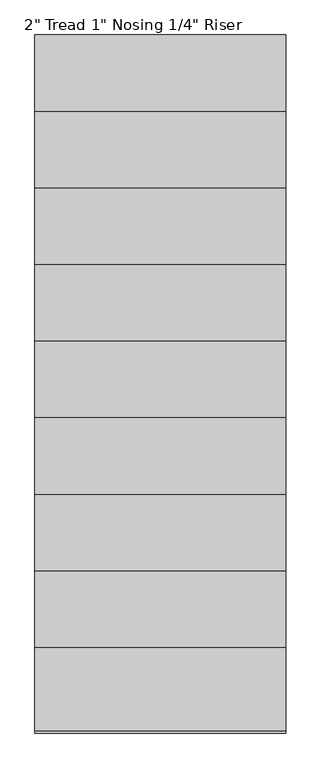
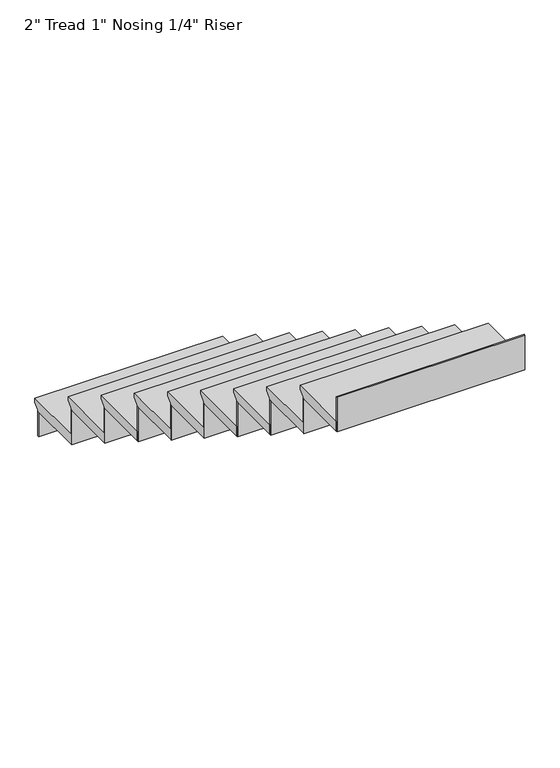
"""IFC4 building model written with IfcOpenShell, lengths in millimetres: stair flight geometry."""

from ifc_helpers import new_model, si_unit, origin, place, context, project, spatial, faceted_brep, source, transform, mapped, element, save


def stair_flight_dc742093(model_context):
    return source(origin(), model_context, "Body", "Brep", [
        faceted_brep([(-3651.3993763, -1023.9064015, 3968.75), (-3651.3993763, -1023.9064015, 3987.8), (-2736.9993763, -1023.9064015, 3987.8), (-2736.9993763, -1023.9064015, 3968.75), (-3651.3993763, -1049.3064015, 3943.35), (-2736.9993763, -1049.3064015, 3943.35), (-3651.3993763, -1328.7064015, 3987.8), (-2736.9993763, -1328.7064015, 3987.8), (-2736.9993763, -1049.3064015, 3937.0), (-2736.9993763, -1328.7064015, 3937.0), (-3651.3993763, -1328.7064015, 3937.0), (-3651.3993763, -1049.3064015, 3937.0)], [[[0, 1, 2, 3]], [[4, 0, 3, 5]], [[2, 1, 6, 7]], [[8, 9, 10, 11]], [[2, 7, 9, 8, 5, 3]], [[8, 11, 4, 5]], [[6, 1, 0, 4, 11, 10]], [[7, 6, 10, 9]]]),
        faceted_brep([(-3651.3993763, -1049.3064015, 3937.0), (-3651.3993763, -1049.3064015, 3810.0), (-3651.3993763, -1055.6564015, 3810.0), (-3651.3993763, -1055.6564015, 3937.0), (-2736.9993763, -1049.3064015, 3937.0), (-2736.9993763, -1055.6564015, 3937.0), (-2736.9993763, -1055.6564015, 3810.0), (-2736.9993763, -1049.3064015, 3810.0)], [[[0, 1, 2, 3]], [[4, 5, 6, 7]], [[1, 0, 4, 7]], [[2, 1, 7, 6]], [[3, 2, 6, 5]], [[0, 3, 5, 4]]]),
        faceted_brep([(-3651.3993763, -1328.7064015, 4114.8), (-3651.3993763, -1328.7064015, 3937.0), (-3651.3993763, -1335.0564015, 3937.0), (-3651.3993763, -1335.0564015, 4114.8), (-2736.9993763, -1328.7064015, 4114.8), (-2736.9993763, -1335.0564015, 4114.8), (-2736.9993763, -1335.0564015, 3937.0), (-2736.9993763, -1328.7064015, 3937.0)], [[[0, 1, 2, 3]], [[4, 5, 6, 7]], [[1, 0, 4, 7]], [[2, 1, 7, 6]], [[3, 2, 6, 5]], [[0, 3, 5, 4]]]),
        faceted_brep([(-2736.9993763, -1303.3064015, 4165.6), (-3651.3993763, -1303.3064015, 4165.6), (-3651.3993763, -1608.1064015, 4165.6), (-2736.9993763, -1608.1064015, 4165.6), (-2736.9993763, -1328.7064015, 4114.8), (-2736.9993763, -1608.1064015, 4114.8), (-3651.3993763, -1608.1064015, 4114.8), (-3651.3993763, -1328.7064015, 4114.8), (-2736.9993763, -1328.7064015, 4121.15), (-2736.9993763, -1303.3064015, 4146.55), (-3651.3993763, -1328.7064015, 4121.15), (-3651.3993763, -1303.3064015, 4146.55)], [[[0, 1, 2, 3]], [[4, 5, 6, 7]], [[0, 3, 5, 4, 8, 9]], [[4, 7, 10, 8]], [[2, 1, 11, 10, 7, 6]], [[3, 2, 6, 5]], [[11, 1, 0, 9]], [[10, 11, 9, 8]]]),
        faceted_brep([(-3651.3993763, -1608.1064015, 4292.6), (-3651.3993763, -1608.1064015, 4114.8), (-3651.3993763, -1614.4564015, 4114.8), (-3651.3993763, -1614.4564015, 4292.6), (-2736.9993763, -1608.1064015, 4292.6), (-2736.9993763, -1614.4564015, 4292.6), (-2736.9993763, -1614.4564015, 4114.8), (-2736.9993763, -1608.1064015, 4114.8)], [[[0, 1, 2, 3]], [[4, 5, 6, 7]], [[1, 0, 4, 7]], [[2, 1, 7, 6]], [[3, 2, 6, 5]], [[0, 3, 5, 4]]]),
        faceted_brep([(-2736.9993763, -1582.7064015, 4343.4), (-3651.3993763, -1582.7064015, 4343.4), (-3651.3993763, -1887.5064015, 4343.4), (-2736.9993763, -1887.5064015, 4343.4), (-2736.9993763, -1608.1064015, 4292.6), (-2736.9993763, -1887.5064015, 4292.6), (-3651.3993763, -1887.5064015, 4292.6), (-3651.3993763, -1608.1064015, 4292.6), (-2736.9993763, -1608.1064015, 4298.95), (-2736.9993763, -1582.7064015, 4324.35), (-3651.3993763, -1608.1064015, 4298.95), (-3651.3993763, -1582.7064015, 4324.35)], [[[0, 1, 2, 3]], [[4, 5, 6, 7]], [[0, 3, 5, 4, 8, 9]], [[4, 7, 10, 8]], [[2, 1, 11, 10, 7, 6]], [[3, 2, 6, 5]], [[11, 1, 0, 9]], [[10, 11, 9, 8]]]),
        faceted_brep([(-3651.3993763, -1887.5064015, 4470.4), (-3651.3993763, -1887.5064015, 4292.6), (-3651.3993763, -1893.8564015, 4292.6), (-3651.3993763, -1893.8564015, 4470.4), (-2736.9993763, -1887.5064015, 4470.4), (-2736.9993763, -1893.8564015, 4470.4), (-2736.9993763, -1893.8564015, 4292.6), (-2736.9993763, -1887.5064015, 4292.6)], [[[0, 1, 2, 3]], [[4, 5, 6, 7]], [[1, 0, 4, 7]], [[2, 1, 7, 6]], [[3, 2, 6, 5]], [[0, 3, 5, 4]]]),
        faceted_brep([(-2736.9993763, -1862.1064015, 4521.2), (-3651.3993763, -1862.1064015, 4521.2), (-3651.3993763, -2166.9064015, 4521.2), (-2736.9993763, -2166.9064015, 4521.2), (-2736.9993763, -1887.5064015, 4470.4), (-2736.9993763, -2166.9064015, 4470.4), (-3651.3993763, -2166.9064015, 4470.4), (-3651.3993763, -1887.5064015, 4470.4), (-2736.9993763, -1887.5064015, 4476.75), (-2736.9993763, -1862.1064015, 4502.15), (-3651.3993763, -1887.5064015, 4476.75), (-3651.3993763, -1862.1064015, 4502.15)], [[[0, 1, 2, 3]], [[4, 5, 6, 7]], [[0, 3, 5, 4, 8, 9]], [[4, 7, 10, 8]], [[2, 1, 11, 10, 7, 6]], [[3, 2, 6, 5]], [[11, 1, 0, 9]], [[10, 11, 9, 8]]]),
        faceted_brep([(-3651.3993763, -2166.9064015, 4648.2), (-3651.3993763, -2166.9064015, 4470.4), (-3651.3993763, -2173.2564015, 4470.4), (-3651.3993763, -2173.2564015, 4648.2), (-2736.9993763, -2166.9064015, 4648.2), (-2736.9993763, -2173.2564015, 4648.2), (-2736.9993763, -2173.2564015, 4470.4), (-2736.9993763, -2166.9064015, 4470.4)], [[[0, 1, 2, 3]], [[4, 5, 6, 7]], [[1, 0, 4, 7]], [[2, 1, 7, 6]], [[3, 2, 6, 5]], [[0, 3, 5, 4]]]),
        faceted_brep([(-2736.9993763, -2141.5064015, 4699.0), (-3651.3993763, -2141.5064015, 4699.0), (-3651.3993763, -2446.3064015, 4699.0), (-2736.9993763, -2446.3064015, 4699.0), (-2736.9993763, -2166.9064015, 4648.2), (-2736.9993763, -2446.3064015, 4648.2), (-3651.3993763, -2446.3064015, 4648.2), (-3651.3993763, -2166.9064015, 4648.2), (-2736.9993763, -2166.9064015, 4654.55), (-2736.9993763, -2141.5064015, 4679.95), (-3651.3993763, -2166.9064015, 4654.55), (-3651.3993763, -2141.5064015, 4679.95)], [[[0, 1, 2, 3]], [[4, 5, 6, 7]], [[0, 3, 5, 4, 8, 9]], [[4, 7, 10, 8]], [[2, 1, 11, 10, 7, 6]], [[3, 2, 6, 5]], [[11, 1, 0, 9]], [[10, 11, 9, 8]]]),
        faceted_brep([(-3651.3993763, -2446.3064015, 4826.0), (-3651.3993763, -2446.3064015, 4648.2), (-3651.3993763, -2452.6564015, 4648.2), (-3651.3993763, -2452.6564015, 4826.0), (-2736.9993763, -2446.3064015, 4826.0), (-2736.9993763, -2452.6564015, 4826.0), (-2736.9993763, -2452.6564015, 4648.2), (-2736.9993763, -2446.3064015, 4648.2)], [[[0, 1, 2, 3]], [[4, 5, 6, 7]], [[1, 0, 4, 7]], [[2, 1, 7, 6]], [[3, 2, 6, 5]], [[0, 3, 5, 4]]]),
        faceted_brep([(-2736.9993763, -2420.9064015, 4876.8), (-3651.3993763, -2420.9064015, 4876.8), (-3651.3993763, -2725.7064015, 4876.8), (-2736.9993763, -2725.7064015, 4876.8), (-2736.9993763, -2446.3064015, 4826.0), (-2736.9993763, -2725.7064015, 4826.0), (-3651.3993763, -2725.7064015, 4826.0), (-3651.3993763, -2446.3064015, 4826.0), (-2736.9993763, -2446.3064015, 4832.35), (-2736.9993763, -2420.9064015, 4857.75), (-3651.3993763, -2446.3064015, 4832.35), (-3651.3993763, -2420.9064015, 4857.75)], [[[0, 1, 2, 3]], [[4, 5, 6, 7]], [[0, 3, 5, 4, 8, 9]], [[4, 7, 10, 8]], [[2, 1, 11, 10, 7, 6]], [[3, 2, 6, 5]], [[11, 1, 0, 9]], [[10, 11, 9, 8]]]),
        faceted_brep([(-3651.3993763, -2725.7064015, 5003.8), (-3651.3993763, -2725.7064015, 4826.0), (-3651.3993763, -2732.0564015, 4826.0), (-3651.3993763, -2732.0564015, 5003.8), (-2736.9993763, -2725.7064015, 5003.8), (-2736.9993763, -2732.0564015, 5003.8), (-2736.9993763, -2732.0564015, 4826.0), (-2736.9993763, -2725.7064015, 4826.0)], [[[0, 1, 2, 3]], [[4, 5, 6, 7]], [[1, 0, 4, 7]], [[2, 1, 7, 6]], [[3, 2, 6, 5]], [[0, 3, 5, 4]]]),
        faceted_brep([(-2736.9993763, -2700.3064015, 5054.6), (-3651.3993763, -2700.3064015, 5054.6), (-3651.3993763, -3005.1064015, 5054.6), (-2736.9993763, -3005.1064015, 5054.6), (-2736.9993763, -2725.7064015, 5003.8), (-2736.9993763, -3005.1064015, 5003.8), (-3651.3993763, -3005.1064015, 5003.8), (-3651.3993763, -2725.7064015, 5003.8), (-2736.9993763, -2725.7064015, 5010.15), (-2736.9993763, -2700.3064015, 5035.55), (-3651.3993763, -2725.7064015, 5010.15), (-3651.3993763, -2700.3064015, 5035.55)], [[[0, 1, 2, 3]], [[4, 5, 6, 7]], [[0, 3, 5, 4, 8, 9]], [[4, 7, 10, 8]], [[2, 1, 11, 10, 7, 6]], [[3, 2, 6, 5]], [[11, 1, 0, 9]], [[10, 11, 9, 8]]]),
        faceted_brep([(-3651.3993763, -3005.1064015, 5181.6), (-3651.3993763, -3005.1064015, 5003.8), (-3651.3993763, -3011.4564015, 5003.8), (-3651.3993763, -3011.4564015, 5181.6), (-2736.9993763, -3005.1064015, 5181.6), (-2736.9993763, -3011.4564015, 5181.6), (-2736.9993763, -3011.4564015, 5003.8), (-2736.9993763, -3005.1064015, 5003.8)], [[[0, 1, 2, 3]], [[4, 5, 6, 7]], [[1, 0, 4, 7]], [[2, 1, 7, 6]], [[3, 2, 6, 5]], [[0, 3, 5, 4]]]),
        faceted_brep([(-2736.9993763, -2979.7064015, 5232.4), (-3651.3993763, -2979.7064015, 5232.4), (-3651.3993763, -3284.5064015, 5232.4), (-2736.9993763, -3284.5064015, 5232.4), (-2736.9993763, -3005.1064015, 5181.6), (-2736.9993763, -3284.5064015, 5181.6), (-3651.3993763, -3284.5064015, 5181.6), (-3651.3993763, -3005.1064015, 5181.6), (-2736.9993763, -3005.1064015, 5187.95), (-2736.9993763, -2979.7064015, 5213.35), (-3651.3993763, -3005.1064015, 5187.95), (-3651.3993763, -2979.7064015, 5213.35)], [[[0, 1, 2, 3]], [[4, 5, 6, 7]], [[0, 3, 5, 4, 8, 9]], [[4, 7, 10, 8]], [[2, 1, 11, 10, 7, 6]], [[3, 2, 6, 5]], [[11, 1, 0, 9]], [[10, 11, 9, 8]]]),
        faceted_brep([(-3651.3993763, -3563.9064015, 5537.2), (-3651.3993763, -3563.9064015, 5359.4), (-3651.3993763, -3570.2564015, 5359.4), (-3651.3993763, -3570.2564015, 5537.2), (-2736.9993763, -3563.9064015, 5537.2), (-2736.9993763, -3570.2564015, 5537.2), (-2736.9993763, -3570.2564015, 5359.4), (-2736.9993763, -3563.9064015, 5359.4)], [[[0, 1, 2, 3]], [[4, 5, 6, 7]], [[1, 0, 4, 7]], [[2, 1, 7, 6]], [[3, 2, 6, 5]], [[0, 3, 5, 4]]]),
        faceted_brep([(-3651.3993763, -3284.5064015, 5359.4), (-3651.3993763, -3284.5064015, 5181.6), (-3651.3993763, -3290.8564015, 5181.6), (-3651.3993763, -3290.8564015, 5359.4), (-2736.9993763, -3284.5064015, 5359.4), (-2736.9993763, -3290.8564015, 5359.4), (-2736.9993763, -3290.8564015, 5181.6), (-2736.9993763, -3284.5064015, 5181.6)], [[[0, 1, 2, 3]], [[4, 5, 6, 7]], [[1, 0, 4, 7]], [[2, 1, 7, 6]], [[3, 2, 6, 5]], [[0, 3, 5, 4]]]),
        faceted_brep([(-2736.9993763, -3563.9064015, 5410.2), (-2736.9993763, -3538.5064015, 5410.2), (-2736.9993763, -3259.1064015, 5410.2), (-3651.3993763, -3259.1064015, 5410.2), (-3651.3993763, -3563.9064015, 5410.2), (-2736.9993763, -3538.5064015, 5359.4), (-2736.9993763, -3563.9064015, 5359.4), (-3651.3993763, -3563.9064015, 5359.4), (-3651.3993763, -3284.5064015, 5359.4), (-2736.9993763, -3284.5064015, 5359.4), (-2736.9993763, -3284.5064015, 5365.75), (-2736.9993763, -3259.1064015, 5391.15), (-3651.3993763, -3284.5064015, 5365.75), (-3651.3993763, -3259.1064015, 5391.15)], [[[0, 1, 2, 3, 4]], [[5, 6, 7, 8, 9]], [[1, 0, 6, 5]], [[2, 1, 5, 9, 10, 11]], [[9, 8, 12, 10]], [[4, 3, 13, 12, 8, 7]], [[0, 4, 7, 6]], [[13, 3, 2, 11]], [[12, 13, 11, 10]]]),
    ])


if __name__ == "__main__":
    model = new_model("IFC4")
    model_context = context("Model", 3, world=origin())
    ifc_project = project(units=[si_unit("LENGTHUNIT", "METRE", prefix="MILLI")], contexts=[model_context])
    site = spatial("IfcSite", under=ifc_project)
    building = spatial("IfcBuilding", under=site)
    placement = place(None, origin())
    stair_flight_shape = stair_flight_dc742093(model_context)
    element("IfcStairFlight", 1, ObjectType="2\" Tread 1\" Nosing 1/4\" Riser", at=placement, inside=building, context=model_context, shape_type="MappedRepresentation", body=[
        mapped(stair_flight_shape, transform((0.0, 0.0, 0.0), x_axis=(1.0, 0.0, 0.0), y_axis=(0.0, 1.0, 0.0), z_axis=(0.0, 0.0, 1.0))),
    ])
    save(model, "model.ifc")
